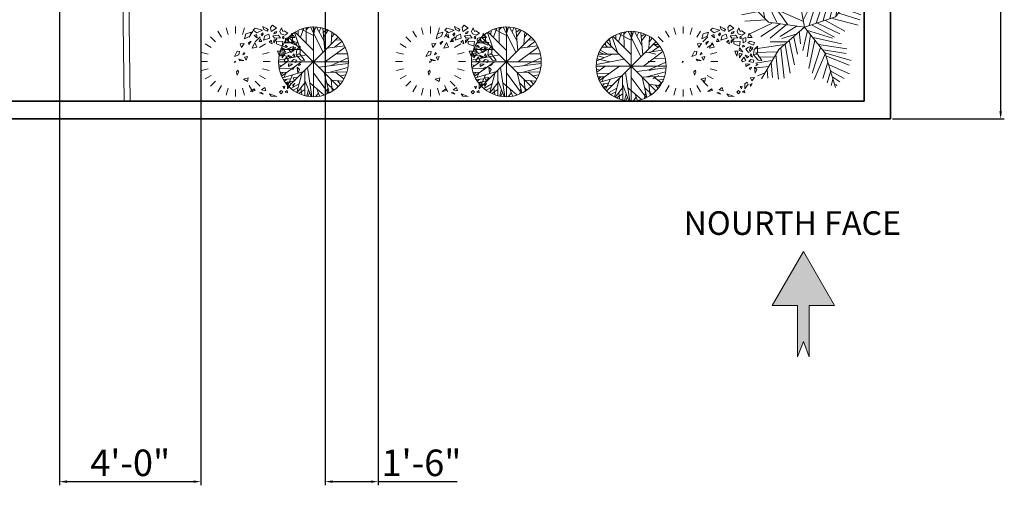
# Model space of a CAD drawing. Units: inches. Extents: x 744 to 1448, y 5126 to 6077.
# Tile 2 of 10: x 1025 to 1359, y 5126 to 5284. Entities that reach past the tile are written whole.
import ezdxf

# ---------------------------------------------------------------- set-up
doc = ezdxf.new("R2010")
doc.units = ezdxf.units.IN
for name, color, linetype, lineweight in [('A-ANNO-DIMS', 2, 'Continuous', 18), ('A-ANNO-SYMB', 7, 'Continuous', 18), ('A-ANNO-TEXT', 7, 'Continuous', 18), ('A-SITE-PVMT', 8, 'Continuous', 18), ('A-WALL', 7, 'Continuous', 35), ('L-PLNT', 3, 'Continuous', 13)]:
    doc.layers.add(name, color=color, linetype=linetype, lineweight=lineweight)
doc.styles.get("Standard").update_dxf_attribs({"font": 'arial.ttf'})
doc.dimstyles.new('ISO-25', dxfattribs={"dimtxt": 9, "dimasz": 2.5, "dimexe": 1.25, "dimexo": 0.625, "dimtad": 1, "dimlunit": 3, "dimtxsty": 'Standard', "dimcen": 2.5, "dimadec": 0, "dimazin": 0, "dimtfac": 1, "dimtmove": 0, "dimatfit": 3, "dimfxl": 1, "dimarcsym": 0})

# ---------------------------------------------------------------- blocks, each defined once
blk = doc.blocks.new('*U10')
for p, q in [((-8.737, 47.138), (-17.069, 52.711)), ((-10.186, 53.64), (-13.084, 55.962)), ((0, 0), (-10.5, 57)), ((-9.099, 51.782), (-6.563, 55.962)), ((-7.288, 39.707), (-21.778, 46.673)), ((-7.65, 43.423), (-2.578, 49.46)), ((-5.839, 35.992), (4.667, 48.067)), ((-5.114, 27.632), (10.463, 46.673)), ((-3.665, 19.273), (-27.574, 35.527)), ((-5.114, 28.097), (-24.676, 40.636)), ((-2.941, 16.486), (8.652, 37.85)), ((27, 9), (48, 36)), ((27.127, 9.056), (31.112, 35.992)), ((44.153, 36.456), (45.239, 32.741)), ((-48.585, 21.131), (-49.309, 29.026)), ((-43.513, 28.561), (-42.427, 15.558)), ((-38.442, 26.239), (-34.819, 7.663)), ((-35.544, 28.097), (-24.314, 3.947)), ((-1.129, 6.734), (9.014, 26.704)), ((10.101, 3.483), (17.708, 26.239)), ((16.259, 5.805), (23.142, 31.348)), ((22.055, 7.198), (27.489, 32.277)), ((31.836, 30.883), (32.561, 16.486)), ((35.096, 32.741), (37.27, 22.524)), ((38.719, 34.134), (41.979, 28.561)), ((40.53, 25.775), (48.862, 24.846)), ((43.791, 29.954), (51.036, 30.883)), ((-47.498, 19.737), (-55.83, 18.344)), ((-31.5, 4.5), (-52.5, 25.5)), ((-14.533, 2.09), (-30.834, 25.31)), ((-24.314, 23.917), (-2.941, 13.7)), ((3.942, 1.625), (11.187, 24.381)), ((36.183, 19.737), (48.137, 17.88)), ((-40.615, 13.7), (-55.105, 10.913)), ((-20.691, 13.7), (-1.129, 4.876)), ((0, 0), (27, 9)), ((29.662, 12.307), (48.137, 6.269)), ((33.285, 16.486), (48.862, 10.913)), ((-33.37, 6.269), (-52.207, 5.34)), ((-28.299, 3.483), (-47.86, -5.805)), ((-21.416, 3.018), (-38.079, -8.128)), ((0, 0), (-31.5, 4.5)), ((-15.982, 2.09), (-30.11, -9.521)), ((0, 0), (-22.5, -19.5)), ((-6.563, 1.161), (-21.416, -8.128)), ((0, 0), (18, -22.5)), ((6.478, 1.625), (26.04, -8.592)), ((11.187, 3.483), (30.749, -5.805)), ((18.07, 5.805), (35.096, -3.483)), ((24.229, 7.663), (46.688, 1.625)), ((-6.563, -5.805), (-19.967, -9.985)), ((-4.752, -3.483), (-3.665, -14.629)), ((2.493, -3.019), (-1.491, -20.202)), ((1.769, -2.555), (24.229, -9.521)), ((5.029, -6.27), (2.131, -25.775)), ((-17.431, -15.094), (-42.789, -18.809)), ((-15.257, -12.772), (-30.11, -12.772)), ((-17.069, -15.094), (-12.721, -40.172)), ((-13.446, -11.378), (-8.737, -32.741)), ((-9.461, -8.592), (-6.201, -23.453)), ((9.014, -11.378), (3.58, -35.992)), ((14.085, -16.951), (6.478, -40.172)), ((7.565, -9.056), (32.198, -14.629)), ((12.274, -15.094), (36.907, -18.809)), ((-24.314, -21.596), (-42.427, -22.06)), ((-22.5, -19.5), (-37.5, -45)), ((-25.038, -23.918), (-22.865, -45.281)), ((-20.691, -18.345), (-17.793, -44.352)), ((18.07, -22.524), (8.289, -45.745)), ((16.259, -19.738), (36.183, -22.989)), ((18, -22.5), (27, -52.5)), ((18.433, -22.524), (40.53, -29.026)), ((19.157, -25.311), (38.719, -33.206)), ((-28.299, -29.026), (-42.789, -31.348)), ((-30.834, -34.135), (-42.427, -35.528)), ((-26.849, -26.24), (-40.253, -25.775)), ((-29.023, -30.884), (-27.936, -43.887)), ((20.244, -30.419), (15.897, -44.816)), ((21.331, -32.741), (39.081, -40.636)), ((-34.457, -39.708), (-40.978, -42.494)), ((-32.646, -36.921), (-31.921, -44.352)), ((22.78, -37.85), (19.519, -48.532)), ((22.78, -38.314), (34.372, -44.816)), ((24.591, -45.745), (23.142, -50.854)), ((24.591, -43.423), (30.749, -47.603)), ((26.764, -49.925), (28.213, -50.854))]:
    blk.add_line(p, q)
blk = doc.blocks.new('*U11')
for points in [[(-5.78, 9.75), (-7.54, 9.23), (-8.01, 7.5), (-6.26, 8.45)], [(-4.43, 11.05), (-5.18, 10.36), (-3.96, 9.49), (-2.07, 10.36)], [(-2, 11.66), (-1.6, 10.62), (-0.52, 10.1), (-0.18, 10.62), (-0.79, 10.96)], [(1.24, 12), (0.56, 11.31), (0.76, 10.01), (2.52, 11.05)], [(2.59, 9.93), (1.84, 9.75), (1.64, 9.23), (2.32, 9.41)], [(4.14, 11.14), (3.6, 10.01), (4, 9.23), (5.22, 8.71), (6.3, 9.41), (5.08, 10.19), (4.61, 10.01)], [(-5.78, 6.81), (-6.66, 6.21), (-6.52, 5.69)], [(-4.84, 8.63), (-3.83, 7.85), (-4.03, 8.97)], [(-2.88, 7.5), (-3.15, 6.64), (-2.27, 6.72)], [(-1.94, 9.49), (-2.48, 8.97), (-2.27, 8.54), (-1.8, 9.06)], [(0.02, 9.06), (-1.33, 8.54), (-1.73, 7.16), (0.29, 7.76)], [(0.76, 7.16), (0.09, 6.46), (1.1, 5.95)], [(1.37, 8.54), (3.13, 8.8), (3.8, 7.85), (1.91, 7.76)], [(1.71, 6.29), (1.71, 7.07), (2.65, 7.5), (2.11, 6.9)], [(2.52, 6.81), (2.52, 5.86), (4.41, 5.17), (4.61, 6.72)], [(4.61, 8.28), (4.54, 7.76), (4.95, 7.59), (4.95, 8.28)], [(6.43, 7.94), (5.49, 7.68), (5.56, 6.21), (6.5, 6.64)], [(7.45, 9.32), (7.11, 7.94), (8.52, 7.94)], [(7.85, 6.81), (7.18, 6.21), (9, 5.51), (9.33, 6.38)], [(-11.32, 1.79), (-9.83, 2.31), (-9.63, 3.44), (-10.44, 3.52)], [(-8.14, 6.03), (-9.36, 5.95), (-9.02, 4.73)], [(-4.57, 6.38), (-5.45, 4.47), (-3.89, 4.82)], [(3.53, 1.88), (2.86, 3.52), (3.8, 3.52)], [(4.41, 4.56), (4.27, 3.7), (5.49, 3.26)], [(5.49, 5.51), (5.42, 4.82), (6.16, 5.08)], [(8.12, 4.99), (7.11, 4.65), (6.5, 4.13), (7.38, 3.09), (8.12, 3.52), (7.65, 3.87)], [(8.73, 4.73), (8.19, 4.56), (8.39, 3.87), (8.59, 4.04)], [(10.28, 5.17), (9.2, 4.04), (9, 2.31), (10.48, 0.49), (11.76, 0.41), (10.35, 2.48), (9.33, 2.4), (10.28, 2.83)], [(-8.21, 0.41), (-9.43, 0.32), (-9.83, 0.84)], [(-8.21, 3.09), (-8.48, 2.31), (-7.87, 2.57)], [(-7, 1.79), (-7.94, 1.53), (-7.47, 0.49)], [(4.27, 2.74), (5.29, 2.66), (4.41, 1.27)], [(5.83, 1.53), (5.02, 0.41), (5.49, -0.02), (6.5, 0.41)], [(7.51, 1.71), (6.91, 1.27), (6.23, 2.14)], [(8.12, 0.75), (7.51, 0.15), (8.93, -0.28), (9.13, 0.49)], [(8.19, 2.57), (7.92, 2.05), (8.66, 1.53)], [(-10.03, -2.71), (-10.64, -3.31), (-10.44, -4.44), (-9.9, -3.49)], [(7.78, -0.8), (6.43, -1.5), (6.43, -0.72)], [(8.32, -1.75), (7.98, -2.53), (7.58, -2.1)], [(9.33, -1.75), (9.54, -3.74), (10.14, -2.53)], [(10.08, -0.63), (9.74, -1.32), (10.48, -0.89)], [(-8.28, -5.73), (-6.79, -5.3), (-7, -6.51)], [(9.33, -5.13), (8.46, -6.25), (7.98, -5.22)], [(-4.84, -8.85), (-4.43, -9.45), (-5.99, -9.8)], [(-2.34, -9.2), (-1.26, -8.5), (-0.99, -9.54)], [(4.07, -9.45), (3.53, -9.97), (4.07, -10.58), (4.61, -9.89)], [(5.29, -7.98), (4.61, -8.16), (5.02, -8.94)], [(6.03, -9.45), (5.42, -9.97), (6.16, -10.15)], [(6.1, -8.94), (6.16, -7.21), (6.91, -6.69), (7.24, -7.38)], [(8.05, -8.07), (8.59, -7.12), (7.92, -7.55)], [(-2.54, -10.06), (-3.02, -10.23), (-1.8, -10.67)], [(0.22, -10.58), (0.83, -11.27), (2.59, -11.36)]]:
    blk.add_lwpolyline(points, close=True)
blk = doc.blocks.new('*U12')
for p, q in [((-25.024, 42.079), (-31.077, 52.563)), ((-13.435, 46.72), (-16.606, 58.557)), ((-1.077, 60.601), (-1.077, 48.601)), ((11.28, 46.72), (14.452, 58.557)), ((22.87, 42.079), (28.923, 52.563)), ((-34.93, 34.454), (-43.503, 43.028)), ((32.776, 34.454), (41.349, 43.028)), ((-42.564, 24.554), (-53.039, 30.601)), ((40.409, 24.554), (50.884, 30.601)), ((-61.077, 0.601), (-49.077, 0.601)), ((-47.5, 13.04), (-59.033, 16.131)), ((45.346, 13.04), (56.878, 16.131)), ((58.923, 0.601), (46.923, 0.601)), ((-47.5, -11.837), (-59.033, -14.928)), ((45.346, -11.837), (56.878, -14.928)), ((-42.564, -23.351), (-53.039, -29.399)), ((-34.93, -33.251), (-43.503, -41.825)), ((32.776, -33.251), (41.349, -41.825)), ((40.409, -23.351), (50.884, -29.399)), ((-25.024, -40.876), (-31.077, -51.36)), ((-13.435, -45.517), (-16.606, -57.354)), ((-1.077, -59.399), (-1.077, -47.399)), ((11.28, -45.517), (14.452, -57.354)), ((22.87, -40.876), (28.923, -51.36))]:
    blk.add_line(p, q)
blk.add_lwpolyline([(-1.908, 0.978), (-2.67, -0.978), (0, 0)], close=True)
blk = doc.blocks.new('*U13')
for p, q in [((-31.2008, 51.1035), (-0.2149, 20.1818)), ((-26.4472, 46.5894), (-26.2712, 53.8116)), ((-22.0458, 42.0753), (-16.5881, 57.6486)), ((-21.1656, 55.8436), (-0.0388, 45.0094)), ((-12.5388, 54.9406), (-7.9613, 59.4546)), ((-12.3627, 32.1443), (-12.5388, 58.7776)), ((-5.3205, 59.6806), (16.5105, 16.7963)), ((2.426, 54.9406), (-1.4472, 59.9056)), ((0, 59.9996), (0, -60)), ((0.4894, 48.6208), (3.6584, 59.6806)), ((18.2711, 35.5298), (5.419, 59.6806)), ((9.8203, 51.5549), (12.8133, 58.5516)), ((19.6795, 19.5047), (16.3344, 57.6486)), ((17.0387, 51.1035), (23.2006, 55.1666)), ((17.7429, 43.6552), (25.4894, 54.2636)), ((31.6513, 50.8778), (30.2429, 30.5643)), ((-45.8134, 38.2383), (-40.5318, 33.0471)), ((-43.8768, 36.4326), (-44.405, 40.2696)), ((42, 42), (-42, -42)), ((42, -42), (-42, 42)), ((-40.1797, 44.558), (-36.4825, 43.2038)), ((-37.0107, 47.0408), (-35.25, 35.5298)), ((-32.6092, 50.4264), (-23.2782, 23.5674)), ((31.1232, 42.5267), (35.8767, 48.1693)), ((36.2288, 25.1474), (48.9049, 35.0784)), ((37.1091, 37.1098), (46.6161, 37.5612)), ((-32.2571, 20.6333), (-59.1937, 9.348)), ((-57.081, 17.9248), (-47.0458, 14.7649)), ((-56.0247, 20.859), (-20.8134, 20.859)), ((-54.7923, 24.4702), (-47.75, 21.0847)), ((-53.2078, 27.4044), (-40.1797, 20.859)), ((-49.8627, 32.8214), (-32.7853, 32.8214)), ((54.3626, 25.3731), (20.9119, 0.3198)), ((23.3767, 23.3417), (53.3063, 27.4044)), ((-59.7219, 2.8025), (-12.0106, 12.0565)), ((-58.6656, 12.7336), (-35.9543, 7.5424)), ((-54.6162, -24.7335), (-20.2853, 0.0941)), ((29.3626, -6.6771), (59.4682, 7.091)), ((38.5175, 13.4107), (58.2359, 13.6364)), ((-60, 0), (60, 0)), ((-59.7219, -4.8714), (-54.2641, -6.6771)), ((-45.2853, -0.1316), (-59.0177, -10.0627)), ((-58.4895, -12.3197), (-36.4825, -11.6426)), ((-53.2078, -27.442), (-16.7641, -16.6081)), ((-14.8275, -15.0282), (-14.6515, -57.6865)), ((-10.074, -10.0627), (-2.5036, -59.7178)), ((9.2922, -9.1598), (59.6443, -2.8401)), ((26.3697, -18.4138), (58.9401, -9.8369)), ((-57.081, -18.4138), (-45.2853, -17.9624)), ((-52.6797, -18.188), (-55.4966, -22.0251)), ((-38.9472, -29.0219), (-51.4472, -30.6018)), ((-47.2219, -19.3166), (-50.2148, -26.3135)), ((-46.5177, -30.1504), (-49.5106, -33.536)), ((-32.4331, -32.4075), (-48.1021, -35.5674)), ((-35.9543, -22.4765), (-44.0529, -40.5329)), ((-19.9331, -20.2194), (-28.5599, -52.721)), ((-14.6515, -32.1818), (-3.912, -59.4922)), ((-0.0388, -19.0909), (25.8415, -53.8495)), ((18.6232, -18.6394), (26.7218, -53.3981)), ((18.7992, -18.6394), (57.3556, -17.2853)), ((30.419, -30.1504), (32.3556, -50.0125)), ((31.4753, -31.279), (49.6091, -33.3103)), ((38.1654, -18.188), (52.426, -29.0219)), ((41.5105, -32.6332), (46.088, -38.0501)), ((45.9119, -24.0564), (55.595, -22.2508)), ((-43.7008, -34.6645), (-46.6937, -37.373)), ((-24.6867, -37.8244), (-38.7712, -45.7241)), ((-26.2712, -43.9185), (-34.7219, -48.6583)), ((-14.6515, -36.2445), (-27.6797, -52.9467)), ((-14.6515, -47.3041), (-25.0388, -54.3009)), ((-21.5177, -45.4984), (-19.9331, -56.1065)), ((-8.4895, -47.5298), (-11.4825, -58.5893)), ((-6.2008, -36.2445), (17.919, -57.0094)), ((5.9471, -46.6269), (10.5246, -58.5893)), ((22.8485, -36.4702), (35.3485, -48.4326)), ((24.7852, -44.8213), (23.0246, -54.978)), ((-6.3768, -52.721), (-9.3698, -58.815)), ((8.4119, -53.1724), (3.8344, -59.4922))]:
    blk.add_line(p, q)
blk.add_circle((0, 0), 60)
blk = doc.blocks.new('*D23')
at = {"layer": 'A-ANNO-DIMS', "color": 0, "lineweight": -2, "transparency": 16777216}
for p, q in [((1321.31, 5821.82), (1359.26, 5821.82)), ((1358.01, 5819.32), (1358.01, 5252.82)), ((1321.31, 5250.32), (1359.26, 5250.32))]:
    blk.add_line(p, q, dxfattribs=at)
at = {"layer": 'A-ANNO-DIMS', "color": 0, "transparency": 16777216}
for points in [[(1357.59, 5819.32), (1358.42, 5819.32), (1358.01, 5821.82)], [(1357.59, 5252.82), (1358.42, 5252.82), (1358.01, 5250.32)]]:
    blk.add_solid(points, dxfattribs=at)
at = {"layer": 'Defpoints', "color": 0, "transparency": 16777216}
for p in [(1320.68, 5821.82), (1320.68, 5250.32), (1358.01, 5250.32)]:
    blk.add_point(p, dxfattribs=at)
at = {"layer": 'A-ANNO-DIMS', "color": 0, "transparency": 16777216, "insert": (1352.81, 5536.07), "char_height": 9, "attachment_point": 5, "rotation": 90}
blk.add_mtext('47\'-7.5"', dxfattribs=at)
blk = doc.blocks.new('*D56')
at = {"layer": 'A-ANNO-DIMS', "color": 0, "lineweight": -2, "transparency": 16777216}
for p, q in [((1038.68, 5750.19), (1038.68, 5125.91)), ((1086.68, 5750.19), (1086.68, 5125.91)), ((1041.18, 5127.16), (1084.18, 5127.16))]:
    blk.add_line(p, q, dxfattribs=at)
at = {"layer": 'A-ANNO-DIMS', "color": 0, "transparency": 16777216}
for points in [[(1041.18, 5127.58), (1041.18, 5126.75), (1038.68, 5127.16)], [(1084.18, 5127.58), (1084.18, 5126.75), (1086.68, 5127.16)]]:
    blk.add_solid(points, dxfattribs=at)
at = {"layer": 'Defpoints', "color": 0, "transparency": 16777216}
for p in [(1038.68, 5750.82), (1086.68, 5750.82), (1086.68, 5127.16)]:
    blk.add_point(p, dxfattribs=at)
at = {"layer": 'A-ANNO-DIMS', "color": 0, "transparency": 16777216, "insert": (1062.68, 5132.38), "char_height": 9, "attachment_point": 5}
blk.add_mtext('4\'-0"', dxfattribs=at)
blk = doc.blocks.new('*D58')
at = {"layer": 'A-ANNO-DIMS', "color": 0, "lineweight": -2, "transparency": 16777216}
for p, q in [((1128.86, 5714.27), (1128.86, 5125.91)), ((1146.83, 5714.27), (1146.83, 5125.91)), ((1131.36, 5127.16), (1144.33, 5127.16)), ((1146.83, 5127.16), (1173.66, 5127.16))]:
    blk.add_line(p, q, dxfattribs=at)
at = {"layer": 'A-ANNO-DIMS', "color": 0, "transparency": 16777216}
for points in [[(1131.36, 5127.58), (1131.36, 5126.75), (1128.86, 5127.16)], [(1144.33, 5127.58), (1144.33, 5126.75), (1146.83, 5127.16)]]:
    blk.add_solid(points, dxfattribs=at)
at = {"layer": 'Defpoints', "color": 0, "transparency": 16777216}
for p in [(1128.86, 5714.9), (1146.83, 5714.9), (1146.83, 5127.16)]:
    blk.add_point(p, dxfattribs=at)
at = {"layer": 'A-ANNO-DIMS', "color": 0, "transparency": 16777216, "insert": (1161.49, 5132.38), "char_height": 9, "attachment_point": 5}
blk.add_mtext('1\'-6"', dxfattribs=at)

msp = doc.modelspace()

# ---------------------------------------------------------------- hatches: boundary and pattern name
at = {"layer": 'A-ANNO-SYMB'}
h = msp.add_hatch(color=256, dxfattribs=at)
h.dxf.hatch_style = 1
h.paths.add_polyline_path([(1291.079, 5205.257), (1280.53, 5186.985), (1289.079, 5186.985), (1289.079, 5169.562), (1291.079, 5174.751), (1293.079, 5169.562), (1293.079, 5186.985), (1301.629, 5186.985)])

# ---------------------------------------------------------------- linework, layer by layer
for p, q in [((1289.079, 5186.985), (1289.079, 5169.562)), ((1293.079, 5186.985), (1293.079, 5169.562)), ((1289.079, 5169.562), (1291.079, 5174.751)), ((1291.079, 5174.751), (1293.079, 5169.562))]:
    msp.add_line(p, q, dxfattribs=at)
msp.add_lwpolyline([(1293.079, 5186.985), (1301.629, 5186.985), (1291.079, 5205.257), (1280.53, 5186.985), (1289.079, 5186.985)], dxfattribs=at)
at = {"layer": 'A-SITE-PVMT'}
for p, q in [((1059.934, 5314.29), (1060.684, 5256.29)), ((1061.934, 5314.316), (1062.684, 5256.316))]:
    msp.add_line(p, q, dxfattribs=at)
at = {"layer": 'A-WALL'}
for p, q in [((1320.684, 5250.316), (1320.684, 5821.816)), ((1311.684, 5256.316), (1311.684, 5314.316)), ((813.684, 5256.316), (1311.684, 5256.316)), ((804.684, 5250.316), (1320.684, 5250.316))]:
    msp.add_line(p, q, dxfattribs=at)

# ---------------------------------------------------------------- block references
at = {"layer": 'L-PLNT'}
for name, p, xscale, yscale, zscale in [('*U10', (1291.509, 5281.439), 0.3894195221065574, 0.3894195221065574, 0.3894195221065574), ('*U11', (1109.7, 5269.687), 1.032484677762128, 1.032484677762128, 1.032484677762128), ('*U11', (1174.728, 5269.687), 1.032484677762128, 1.032484677762128, 1.032484677762128), ('*U11', (1264.871, 5269.687), 1.032484677762128, 1.032484677762128, 1.032484677762128), ('*U12', (1098.564, 5269.687), 0.1976487053468327, 0.1976487053468327, 0.1976487053468327), ('*U13', (1124.855, 5269.687), 0.1976487053468327, 0.1976487053468327, 0.1976487053468327), ('*U12', (1164.756, 5269.687), 0.1976487053468327, 0.1976487053468327, 0.1976487053468327), ('*U13', (1190.314, 5269.687), 0.1976487053468327, 0.1976487053468327, 0.1976487053468327), ('*U13', (1232.666, 5268.175), 0.1976487053468327, 0.1976487053468327, 0.1976487053468327), ('*U12', (1250.466, 5269.687), 0.1976487053468327, 0.1976487053468327, 0.1976487053468327)]:
    msp.add_blockref(name, p, dxfattribs=dict(at, xscale=xscale, yscale=yscale, zscale=zscale))

# ---------------------------------------------------------------- texts
at = {"layer": 'A-ANNO-TEXT', "insert": (1250.444, 5218.936), "char_height": 8, "attachment_point": 1}
msp.add_mtext_dynamic_manual_height_columns('NOURTH FACE', width=83.5941, gutter_width=12.5, heights=[0], dxfattribs=at)

# ---------------------------------------------------------------- dimensions: what is measured, and where the dimension line sits
at = {"layer": 'A-ANNO-DIMS'}
dim = msp.add_linear_dim(base=(1358.008, 5250.316), p1=(1320.684, 5821.816), p2=(1320.684, 5250.316), angle=90, dimstyle='ISO-25', override={"dimclrd": 0, "dimclre": 0, "dimclrt": 0}, dxfattribs=at)
dim.commit()
dim.dimension.update_dxf_attribs({"geometry": '*D23', "text_midpoint": (1352.806, 5536.066)})
for base, p1, p2, picture, middle in [((1086.684, 5127.162), (1038.684, 5750.816), (1086.684, 5750.816), '*D56', (1062.684, 5132.383)), ((1146.829, 5127.162), (1128.864, 5714.896), (1146.829, 5714.896), '*D58', (1161.493, 5132.383))]:
    dim = msp.add_linear_dim(base=base, p1=p1, p2=p2, dimstyle='ISO-25', override={"dimdec": 1, "dimlfac": 1, "dimrnd": 0, "dimzin": 1, "dimdsep": 46, "dimlunit": 4, "dimfrac": 2}, dxfattribs=at)
    dim.commit()
    dim.dimension.update_dxf_attribs({"geometry": picture, "text_midpoint": middle})

doc.saveas('drawing.dxf')
